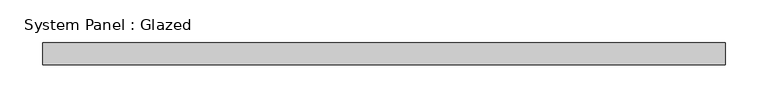
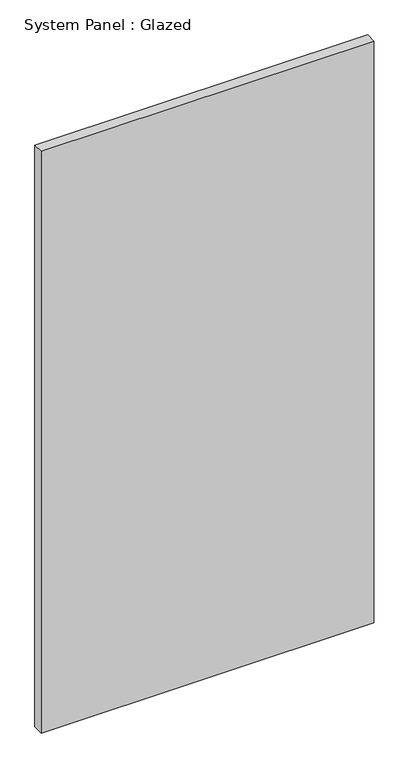
"""IFC4 building model written with IfcOpenShell, lengths in millimetres: plate geometry, System Panel : Glazed."""

from ifc_helpers import new_model, si_unit, origin, origin_with_axes, place, context, project, spatial, polyline, outline, extrude, source, transform, mapped, element, save


def system_panel_glazed_89fef50d(model_context):
    return source(origin(), model_context, "Body", "SweptSolid", [
        extrude(outline(polyline([(396.875, 19.05), (-396.875, 19.05), (-396.875, 44.45), (396.875, 44.45), (396.875, 19.05)])), origin_with_axes(), (0.0, 0.0, 1.0), 1467.6445261),
    ])


if __name__ == "__main__":
    model = new_model("IFC4")
    model_context = context("Model", 3, world=origin())
    ifc_project = project(units=[si_unit("LENGTHUNIT", "METRE", prefix="MILLI")], contexts=[model_context])
    site = spatial("IfcSite", under=ifc_project)
    building = spatial("IfcBuilding", under=site)
    placement = place(None, origin())
    system_panel_glazed_shape = system_panel_glazed_89fef50d(model_context)
    element("IfcPlate", 1, ObjectType="System Panel : Glazed", at=placement, inside=building, context=model_context, shape_type="MappedRepresentation", body=[
        mapped(system_panel_glazed_shape, transform((0.0, 0.0, 0.0), x_axis=(1.0, 0.0, 0.0), y_axis=(0.0, 1.0, 0.0), z_axis=(0.0, 0.0, 1.0))),
    ])
    save(model, "model.ifc")

# Revit data of these elements
# Type "System Panel : Glazed"
#   Construction Type Id = "GSP4R"
#   Analytic Construction = "1/8 in Pilkington single glazing"
#   Visual Light Transmittance = 0.9
#   Solar Heat Gain Coefficient = 0.86
#   Heat Transfer Coefficient (U) = 1.18115 BTU/(h·ft²·°F)
#   Define Thermal Properties by = 1
# Element 1 (IfcPlate, "System Panel : Glazed")
#   Materials on its faces: "Glass"
# Materials
#   "Glass": class "Glass", colour RGB 0 128 192, transparency 0.75, Description = "Soda Lime Glass", Cost = 0
